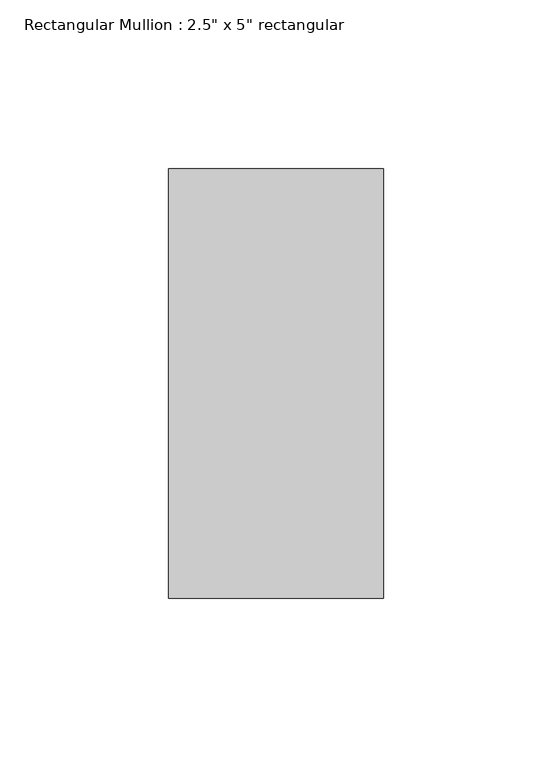
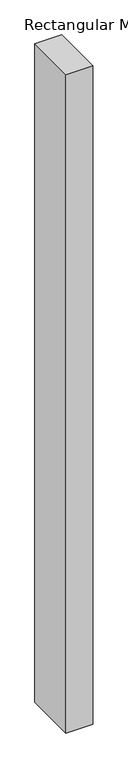
"""IFC4 building model written with IfcOpenShell, lengths in millimetres: member geometry."""

from ifc_helpers import new_model, si_unit, frame, origin, place, context, project, spatial, polyline, outline, extrude, source, transform, mapped, element, save


def member_ea29af33(model_context):
    return source(origin(), model_context, "Body", "SweptSolid", [
        extrude(outline(polyline([(0.0, 63.5), (0.0, -63.5), (-63.5, -63.5), (-63.5, 63.5), (0.0, 63.5)])), frame((0.0, 0.0, -1646.9538703), z_axis=(0.0, 0.0, 1.0), x_axis=(1.0, 0.0, 0.0)), (0.0, 0.0, 1.0), 1646.9538703),
    ])


if __name__ == "__main__":
    model = new_model("IFC4")
    model_context = context("Model", 3, world=origin())
    ifc_project = project(units=[si_unit("LENGTHUNIT", "METRE", prefix="MILLI")], contexts=[model_context])
    site = spatial("IfcSite", under=ifc_project)
    building = spatial("IfcBuilding", under=site)
    placement = place(None, origin())
    member_shape = member_ea29af33(model_context)
    element("IfcMember", 1, ObjectType="Rectangular Mullion : 2.5\" x 5\" rectangular", at=placement, inside=building, context=model_context, shape_type="MappedRepresentation", body=[
        mapped(member_shape, transform((0.0, 0.0, 0.0), x_axis=(1.0, 0.0, 0.0), y_axis=(0.0, 1.0, 0.0), z_axis=(0.0, 0.0, 1.0))),
    ])
    save(model, "model.ifc")

# Revit data of these elements
# Type "Rectangular Mullion : 2.5\" x 5\" rectangular"
#   built-in parameter 1007304 = 0.416667 (stored number, unit not read)
#   built-in parameter 1007301 = 0.104167 (stored number, unit not read)
#   built-in parameter 1007300 = 0.104167 (stored number, unit not read)
# Element 1 (IfcMember, "Rectangular Mullion : 2.5\" x 5\" rectangular")
#   Materials on its faces: "Aluminum"
# Materials
#   "Aluminum": class "Metal", colour RGB 247 247 247, transparency 0, Description = "Aluminum 6061", Cost = 0
